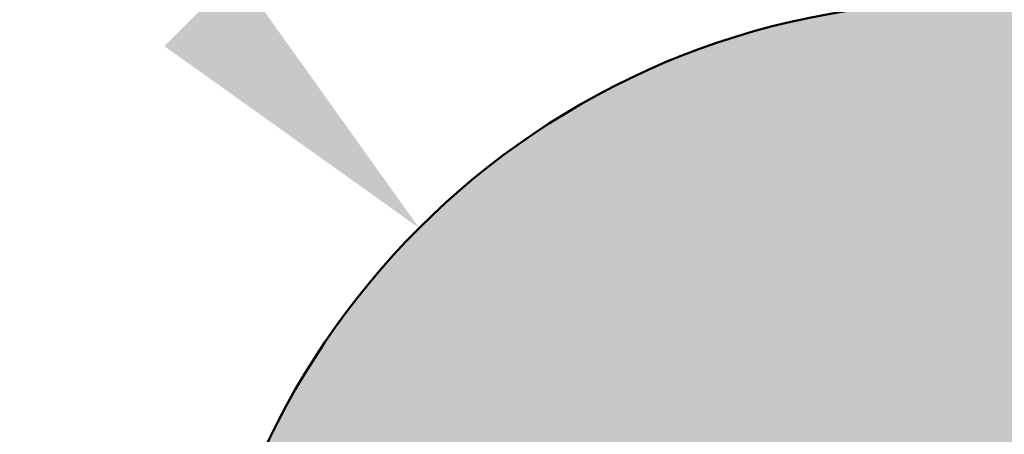
# Model space of a CAD drawing. Units: millimetres. Extents: x 0 to 2267, y 0 to 1823.
# Tile 15 of 256: x 1518.68 to 1531.44, y 1121.82 to 1127.19. Entities that reach past the tile are written whole.
import ezdxf

# ---------------------------------------------------------------- set-up
doc = ezdxf.new("R2010")
doc.units = ezdxf.units.MM
doc.header["$MEASUREMENT"] = 0
for name, color, linetype, lineweight in [('M-DIMS', 2, 'Continuous', 25), ('M-HATC', 252, 'Continuous', 18), ('M-OUTL', 7, 'Continuous', 50)]:
    doc.layers.add(name, color=color, linetype=linetype, lineweight=lineweight)
doc.styles.get("Standard").update_dxf_attribs({"font": 'arial.ttf'})
doc.dimstyles.get("Standard").update_dxf_attribs({"dimtxt": 7, "dimasz": 4, "dimexe": 0.18, "dimexo": 0.0625, "dimgap": 0.09, "dimtad": 0, "dimdec": 0, "dimzin": 0, "dimdsep": 46, "dimtxsty": 'Standard', "dimcen": 0.09, "dimadec": 0, "dimazin": 0, "dimtfac": 1, "dimtdec": 0, "dimtofl": 0, "dimtmove": 0, "dimatfit": 3, "dimfxl": 1, "dimtolj": 1, "dimtzin": 0, "dimarcsym": 0})

# ---------------------------------------------------------------- blocks, each defined once
blk = doc.blocks.new('*D28')
at = {"layer": 'Defpoints', "color": 0, "transparency": 16777216}
for p in [(1523.858, 1124.488), (1530.929, 1117.417)]:
    blk.add_point(p, dxfattribs=at)
at = {"layer": 'M-DIMS', "color": 0, "lineweight": -2, "transparency": 16777216}
for p, q in [((1518.201, 1130.145), (1521.029, 1127.317)), ((1530.839, 1117.417), (1531.019, 1117.417)), ((1530.929, 1117.327), (1530.929, 1117.507))]:
    blk.add_line(p, q, dxfattribs=at)
at = {"layer": 'M-DIMS', "color": 0, "transparency": 16777216}
blk.add_solid([(1521.501, 1127.788), (1520.558, 1126.845), (1523.858, 1124.488)], dxfattribs=at)
at = {"layer": 'M-DIMS', "color": 0, "transparency": 16777216, "insert": (1504.949, 1143.397), "char_height": 7, "attachment_point": 5, "rotation": 314.9998}
blk.add_mtext('\\A1;27X R10', dxfattribs=at)

msp = doc.modelspace()

# ---------------------------------------------------------------- hatches: boundary and pattern name
at = {"layer": 'M-HATC'}
h = msp.add_hatch(color=256, dxfattribs=at)
h.dxf.hatch_style = 1
h.paths.add_polyline_path([(2055.771, 1603.062), (1381.087, 1603.062), (1381.087, 1598.062), (2055.771, 1598.062)])
h.paths.add_polyline_path([(2055.771, 1598.062), (1381.087, 1598.062), (1381.087, 1593.062), (2055.771, 1593.062)])
h.paths.add_polyline_path([(2051.307, 1536.761), (1385.55, 1536.761), (1385.55, 1526.761), (1387.55, 1526.761), (1388.537, 1525.053), (1385.332, 1521.233), (1385.332, 1521.223), (2050.254, 1522.749), (2048.321, 1525.053), (2049.307, 1526.761), (2051.307, 1526.761)])
edge = h.paths.add_edge_path()
edge.add_arc((1847.535, 1379.149), 135, 222.60306, 222.89085, ccw=False)
edge.add_line((1748.166, 1287.766), (1683.092, 1287.766))
edge.add_arc((1583.724, 1379.149), 135, 317.10915, 317.39694, ccw=False)
edge.add_arc((1678.969, 1290.671), 5, 222.8909, 317.1091, ccw=False)
edge.add_arc((1774.213, 1379.149), 135, 222.60306, 222.89085, ccw=False)
edge.add_line((1674.845, 1287.766), (1609.771, 1287.766))
edge.add_arc((1510.403, 1379.149), 135, 317.10915, 317.39694, ccw=False)
edge.add_arc((1605.647, 1290.671), 5, 222.8909, 317.1091, ccw=False)
edge.add_arc((1700.892, 1379.149), 135, 222.60306, 222.89085, ccw=False)
edge.add_line((1601.524, 1287.766), (1536.45, 1287.766))
edge.add_arc((1437.081, 1379.149), 135, 317.10915, 317.39694, ccw=False)
edge.add_arc((1532.326, 1290.671), 5, 222.8909, 317.1091, ccw=False)
edge.add_arc((1627.571, 1379.149), 135, 222.60306, 222.89085, ccw=False)
edge.add_line((1528.203, 1287.766), (1505.929, 1287.766))
edge.add_spline(control_points=[(1505.929, 1287.766), (1504.262, 1287.766), (1504.262, 1282.766), (1505.929, 1282.766)], knot_values=[0, 0, 0, 0, 5, 5, 5, 5], degree=3, periodic=0)
edge.add_line((1505.929, 1282.766), (1930.929, 1282.766))
edge.add_spline(control_points=[(1930.929, 1282.766), (1932.596, 1282.766), (1932.596, 1287.766), (1930.929, 1287.766)], knot_values=[0, 0, 0, 0, 5, 5, 5, 5], degree=3, periodic=0)
edge.add_line((1930.929, 1287.766), (1903.056, 1287.766))
edge.add_arc((1803.688, 1379.149), 135, 317.10915, 317.39694, ccw=False)
edge.add_arc((1898.932, 1290.671), 5, 222.8909, 317.1091, ccw=False)
edge.add_arc((1994.177, 1379.149), 135, 222.60306, 222.89085, ccw=False)
edge.add_line((1894.809, 1287.766), (1829.735, 1287.766))
edge.add_arc((1730.366, 1379.149), 135, 317.10915, 317.39694, ccw=False)
edge.add_arc((1825.611, 1290.671), 5, 222.8909, 317.1091, ccw=False)
edge.add_arc((1920.856, 1379.149), 135, 222.60306, 222.89085, ccw=False)
edge.add_line((1821.487, 1287.766), (1756.413, 1287.766))
edge.add_arc((1657.045, 1379.149), 135, 317.10915, 317.39694, ccw=False)
edge.add_arc((1752.29, 1290.671), 5, 222.8909, 317.1091, ccw=False)
edge = h.paths.add_edge_path()
edge.add_spline(control_points=[(1843.429, 1227.247), (1845.096, 1227.247), (1845.096, 1232.247), (1843.429, 1232.247)], knot_values=[0, 0, 0, 0, 5, 5, 5, 5], degree=3, periodic=0)
edge.add_line((1843.429, 1232.247), (1593.429, 1232.247))
edge.add_spline(control_points=[(1593.429, 1232.247), (1591.762, 1232.247), (1591.762, 1227.247), (1593.429, 1227.247)], knot_values=[0, 0, 0, 0, 5, 5, 5, 5], degree=3, periodic=0)
edge.add_line((1593.429, 1227.247), (1843.429, 1227.247))
h.paths.add_polyline_path([(1905.929, 1127.417), (1530.929, 1127.417, 0.414214), (1520.929, 1117.417), (1530.929, 1117.417), (1915.929, 1117.417, 0.414214)])
edge = h.paths.add_edge_path()
edge.add_arc((1397.086, 1498.408), 12.73, 90.7821, 190.8787, ccw=False)
edge.add_line((1396.912, 1511.136), (1428.01, 1511.349))
edge.add_line((1428.01, 1511.349), (1433.01, 1511.349))
edge.add_line((1433.01, 1511.349), (1434.439, 1511.349))
edge.add_arc((1419.474, 1498.08), 20, 41.561, 74.0821)
edge.add_line((1424.959, 1517.314), (1399.935, 1517.256))
edge.add_spline(control_points=[(1399.931, 1517.256), (1399.884, 1517.213), (1399.833, 1517.169), (1399.777, 1517.124)], knot_values=[11.567499, 11.567499, 11.567499, 11.567499, 11.814249, 11.814249, 11.814249, 11.814249], degree=3, periodic=0)
edge.add_spline(control_points=[(1399.633, 1517.01), (1399.583, 1516.972), (1399.531, 1516.934), (1399.476, 1516.895)], knot_values=[11.167718, 11.167718, 11.167718, 11.167718, 11.365188, 11.365188, 11.365188, 11.365188], degree=3, periodic=0)
edge.add_spline(control_points=[(1399.34, 1516.8), (1399.151, 1516.672), (1398.938, 1516.538), (1398.704, 1516.399)], knot_values=[10.376405, 10.376405, 10.376405, 10.376405, 11.00994, 11.00994, 11.00994, 11.00994], degree=3, periodic=0)
edge.add_spline(control_points=[(1398.657, 1516.372), (1398.579, 1516.326), (1398.498, 1516.28), (1398.415, 1516.233)], knot_values=[10.125175, 10.125175, 10.125175, 10.125175, 10.334406, 10.334406, 10.334406, 10.334406], degree=3, periodic=0)
edge.add_spline(control_points=[(1398.264, 1516.149), (1398.196, 1516.111), (1398.126, 1516.073), (1398.055, 1516.035)], knot_values=[9.832246, 9.832246, 9.832246, 9.832246, 9.999658, 9.999658, 9.999658, 9.999658], degree=3, periodic=0)
edge.add_spline(control_points=[(1397.999, 1516.005), (1397.731, 1515.862), (1397.446, 1515.717), (1397.147, 1515.571)], knot_values=[9.161808, 9.161808, 9.161808, 9.161808, 9.787769, 9.787769, 9.787769, 9.787769], degree=3, periodic=0)
edge.add_spline(control_points=[(1397.147, 1515.571), (1396.842, 1515.423), (1396.522, 1515.274), (1396.191, 1515.126)], knot_values=[8.524455, 8.524455, 8.524455, 8.524455, 9.161808, 9.161808, 9.161808, 9.161808], degree=3, periodic=0)
edge.add_spline(control_points=[(1396.078, 1515.076), (1395.985, 1515.035), (1395.892, 1514.994), (1395.798, 1514.953)], knot_values=[8.275193, 8.275193, 8.275193, 8.275193, 8.451726, 8.451726, 8.451726, 8.451726], degree=3, periodic=0)
edge.add_spline(control_points=[(1395.602, 1514.869), (1395.5, 1514.826), (1395.397, 1514.782), (1395.293, 1514.739)], knot_values=[7.962917, 7.962917, 7.962917, 7.962917, 8.152764, 8.152764, 8.152764, 8.152764], degree=3, periodic=0)
edge.add_spline(control_points=[(1395.212, 1514.706), (1394.828, 1514.547), (1394.435, 1514.393), (1394.036, 1514.244)], knot_values=[7.21254, 7.21254, 7.21254, 7.21254, 7.913148, 7.913148, 7.913148, 7.913148], degree=3, periodic=0)
edge.add_spline(control_points=[(1394.036, 1514.244), (1393.708, 1514.121), (1393.375, 1514.003), (1393.043, 1513.889)], knot_values=[6.633733, 6.633733, 6.633733, 6.633733, 7.21254, 7.21254, 7.21254, 7.21254], degree=3, periodic=0)
edge.add_spline(control_points=[(1392.821, 1513.815), (1392.72, 1513.781), (1392.618, 1513.748), (1392.517, 1513.715)], knot_values=[6.328796, 6.328796, 6.328796, 6.328796, 6.505493, 6.505493, 6.505493, 6.505493], degree=3, periodic=0)
edge.add_spline(control_points=[(1392.517, 1513.715), (1392.319, 1513.652), (1392.121, 1513.59), (1391.924, 1513.531)], knot_values=[5.984605, 5.984605, 5.984605, 5.984605, 6.328796, 6.328796, 6.328796, 6.328796], degree=3, periodic=0)
edge.add_spline(control_points=[(1391.792, 1513.491), (1391.312, 1513.35), (1390.838, 1513.224), (1390.378, 1513.117)], knot_values=[5.066697, 5.066697, 5.066697, 5.066697, 5.907055, 5.907055, 5.907055, 5.907055], degree=3, periodic=0)
edge.add_spline(control_points=[(1390.378, 1513.117), (1390.18, 1513.071), (1389.984, 1513.028), (1389.791, 1512.99)], knot_values=[4.70367, 4.70367, 4.70367, 4.70367, 5.066695, 5.066695, 5.066695, 5.066695], degree=3, periodic=0)
edge.add_spline(control_points=[(1389.422, 1512.92), (1389.246, 1512.889), (1389.073, 1512.862), (1388.904, 1512.838)], knot_values=[4.130571, 4.130571, 4.130571, 4.130571, 4.469816, 4.469816, 4.469816, 4.469816], degree=3, periodic=0)
edge.add_spline(control_points=[(1388.904, 1512.838), (1388.591, 1512.795), (1388.291, 1512.764), (1388.007, 1512.749)], knot_values=[3.504031, 3.504031, 3.504031, 3.504031, 4.130571, 4.130571, 4.130571, 4.130571], degree=3, periodic=0)
edge.add_spline(control_points=[(1387.936, 1512.746), (1387.854, 1512.742), (1387.773, 1512.74), (1387.694, 1512.739)], knot_values=[3.268866, 3.268866, 3.268866, 3.268866, 3.451164, 3.451164, 3.451164, 3.451164], degree=3, periodic=0)
edge.add_spline(control_points=[(1387.335, 1512.744), (1387.208, 1512.75), (1387.085, 1512.76), (1386.967, 1512.774)], knot_values=[2.670686, 2.670686, 2.670686, 2.670686, 2.984, 2.984, 2.984, 2.984], degree=3, periodic=0)
edge.add_spline(control_points=[(1386.833, 1512.792), (1386.821, 1512.794), (1386.809, 1512.796), (1386.797, 1512.798)], knot_values=[2.516981, 2.516981, 2.516981, 2.516981, 2.549528, 2.549528, 2.549528, 2.549528], degree=3, periodic=0)
edge.add_spline(control_points=[(1386.453, 1512.873), (1386.426, 1512.881), (1386.399, 1512.889), (1386.373, 1512.897)], knot_values=[2.095869, 2.095869, 2.095869, 2.095869, 2.17941, 2.17941, 2.17941, 2.17941], degree=3, periodic=0)
edge.add_spline(control_points=[(1386.069, 1513.019), (1386.063, 1513.022), (1386.058, 1513.025), (1386.052, 1513.028)], knot_values=[1.72453, 1.72453, 1.72453, 1.72453, 1.745933, 1.745933, 1.745933, 1.745933], degree=3, periodic=0)
edge.add_arc((1399.474, 1498.08), 20, 131.8243, 180)
edge.add_arc((1630.334, 1505.548), 250.971, 181.70518, 236.42798)
edge.add_arc((1605.34, 1483.304), 218.782, 238.66083, 243.34961)
edge.add_arc((1647.091, 1510.359), 262.899, 183.12984, 237.85344, ccw=False)
h.paths.add_polyline_path([(1406.537, 1391.964, 0.149382), (1491.551, 1296.442, -0.129517)], flags=17)
edge = h.paths.add_edge_path()
edge.add_arc((2037.384, 1498.08), 20, 0, 48.2659)
edge.add_spline(control_points=[(2050.697, 1513.005), (2050.651, 1512.985), (2050.603, 1512.966), (2050.554, 1512.948)], knot_values=[1.835652, 1.835652, 1.835652, 1.835652, 2.000781, 2.000781, 2.000781, 2.000781], degree=3, periodic=0)
edge.add_spline(control_points=[(2050.462, 1512.917), (2050.479, 1512.922), (2050.496, 1512.928), (2050.513, 1512.934)], knot_values=[2.045477, 2.045477, 2.045477, 2.045477, 2.101389, 2.101389, 2.101389, 2.101389], degree=3, periodic=0)
edge.add_spline(control_points=[(2050.129, 1512.834), (2050.198, 1512.847), (2050.266, 1512.862), (2050.331, 1512.879)], knot_values=[2.237629, 2.237629, 2.237629, 2.237629, 2.435841, 2.435841, 2.435841, 2.435841], degree=3, periodic=0)
edge.add_spline(control_points=[(2050.095, 1512.828), (2050.106, 1512.83), (2050.118, 1512.832), (2050.129, 1512.834)], knot_values=[2.435841, 2.435841, 2.435841, 2.435841, 2.468321, 2.468321, 2.468321, 2.468321], degree=3, periodic=0)
edge.add_spline(control_points=[(2049.784, 1512.785), (2049.855, 1512.792), (2049.924, 1512.801), (2049.992, 1512.811)], knot_values=[2.563852, 2.563852, 2.563852, 2.563852, 2.748541, 2.748541, 2.748541, 2.748541], degree=3, periodic=0)
edge.add_spline(control_points=[(2049.405, 1512.762), (2049.536, 1512.765), (2049.663, 1512.773), (2049.784, 1512.785)], knot_values=[2.748541, 2.748541, 2.748541, 2.748541, 3.064882, 3.064882, 3.064882, 3.064882], degree=3, periodic=0)
edge.add_spline(control_points=[(2049.17, 1512.76), (2049.234, 1512.759), (2049.297, 1512.759), (2049.358, 1512.761)], knot_values=[3.102309, 3.102309, 3.102309, 3.102309, 3.2503, 3.2503, 3.2503, 3.2503], degree=3, periodic=0)
edge.add_spline(control_points=[(2048.857, 1512.769), (2048.964, 1512.764), (2049.068, 1512.761), (2049.17, 1512.76)], knot_values=[3.2503, 3.2503, 3.2503, 3.2503, 3.486069, 3.486069, 3.486069, 3.486069], degree=3, periodic=0)
edge.add_spline(control_points=[(2048.692, 1512.779), (2048.373, 1512.801), (2048.035, 1512.841), (2047.682, 1512.897)], knot_values=[3.606429, 3.606429, 3.606429, 3.606429, 4.2989, 4.2989, 4.2989, 4.2989], degree=3, periodic=0)
edge.add_spline(control_points=[(2047.682, 1512.897), (2047.546, 1512.919), (2047.408, 1512.942), (2047.268, 1512.969)], knot_values=[4.2989, 4.2989, 4.2989, 4.2989, 4.565769, 4.565769, 4.565769, 4.565769], degree=3, periodic=0)
edge.add_spline(control_points=[(2047.268, 1512.969), (2047.145, 1512.991), (2047.021, 1513.016), (2046.895, 1513.042)], knot_values=[4.565769, 4.565769, 4.565769, 4.565769, 4.799971, 4.799971, 4.799971, 4.799971], degree=3, periodic=0)
edge.add_spline(control_points=[(2046.895, 1513.042), (2046.529, 1513.119), (2046.151, 1513.209), (2045.768, 1513.311)], knot_values=[4.799971, 4.799971, 4.799971, 4.799971, 5.483718, 5.483718, 5.483718, 5.483718], degree=3, periodic=0)
edge.add_spline(control_points=[(2045.768, 1513.311), (2045.372, 1513.415), (2044.97, 1513.532), (2044.566, 1513.659)], knot_values=[5.483718, 5.483718, 5.483718, 5.483718, 6.187866, 6.187866, 6.187866, 6.187866], degree=3, periodic=0)
edge.add_spline(control_points=[(2044.566, 1513.659), (2044.415, 1513.706), (2044.263, 1513.755), (2044.112, 1513.805)], knot_values=[6.187866, 6.187866, 6.187866, 6.187866, 6.451551, 6.451551, 6.451551, 6.451551], degree=3, periodic=0)
edge.add_spline(control_points=[(2044.112, 1513.805), (2043.997, 1513.843), (2043.882, 1513.881), (2043.767, 1513.92)], knot_values=[6.451551, 6.451551, 6.451551, 6.451551, 6.651434, 6.651434, 6.651434, 6.651434], degree=3, periodic=0)
edge.add_spline(control_points=[(2043.767, 1513.92), (2043.372, 1514.055), (2042.977, 1514.198), (2042.589, 1514.346)], knot_values=[6.651434, 6.651434, 6.651434, 6.651434, 7.338879, 7.338879, 7.338879, 7.338879], degree=3, periodic=0)
edge.add_spline(control_points=[(2042.589, 1514.346), (2042.164, 1514.507), (2041.746, 1514.675), (2041.341, 1514.846)], knot_values=[7.338879, 7.338879, 7.338879, 7.338879, 8.089209, 8.089209, 8.089209, 8.089209], degree=3, periodic=0)
edge.add_spline(control_points=[(2041.341, 1514.846), (2041.103, 1514.946), (2040.869, 1515.048), (2040.64, 1515.15)], knot_values=[8.089209, 8.089209, 8.089209, 8.089209, 8.529587, 8.529587, 8.529587, 8.529587], degree=3, periodic=0)
edge.add_spline(control_points=[(2040.51, 1515.209), (2040.082, 1515.402), (2039.675, 1515.597), (2039.295, 1515.789)], knot_values=[8.613818, 8.613818, 8.613818, 8.613818, 9.44571, 9.44571, 9.44571, 9.44571], degree=3, periodic=0)
edge.add_spline(control_points=[(2039.295, 1515.789), (2039.062, 1515.907), (2038.839, 1516.025), (2038.629, 1516.14)], knot_values=[9.44571, 9.44571, 9.44571, 9.44571, 9.956404, 9.956404, 9.956404, 9.956404], degree=3, periodic=0)
edge.add_spline(control_points=[(2038.629, 1516.14), (2038.519, 1516.2), (2038.412, 1516.26), (2038.309, 1516.319)], knot_values=[9.956404, 9.956404, 9.956404, 9.956404, 10.223542, 10.223542, 10.223542, 10.223542], degree=3, periodic=0)
edge.add_spline(control_points=[(2038.309, 1516.319), (2038.214, 1516.374), (2038.122, 1516.428), (2038.033, 1516.481)], knot_values=[10.223542, 10.223542, 10.223542, 10.223542, 10.47051, 10.47051, 10.47051, 10.47051], degree=3, periodic=0)
edge.add_spline(control_points=[(2038.033, 1516.481), (2037.786, 1516.63), (2037.564, 1516.773), (2037.372, 1516.909)], knot_values=[10.47051, 10.47051, 10.47051, 10.47051, 11.15767, 11.15767, 11.15767, 11.15767], degree=3, periodic=0)
edge.add_spline(control_points=[(2037.372, 1516.909), (2037.279, 1516.975), (2037.193, 1517.04), (2037.114, 1517.102)], knot_values=[11.15767, 11.15767, 11.15767, 11.15767, 11.49227, 11.49227, 11.49227, 11.49227], degree=3, periodic=0)
edge.add_spline(control_points=[(2036.856, 1517.326), (2036.915, 1517.269), (2036.981, 1517.21), (2037.056, 1517.149)], knot_values=[11.577341, 11.577341, 11.577341, 11.577341, 11.91035, 11.91035, 11.91035, 11.91035], degree=3, periodic=0)
edge.add_spline(control_points=[(2036.807, 1517.375), (2036.823, 1517.359), (2036.839, 1517.342), (2036.856, 1517.326)], knot_values=[11.91035, 11.91035, 11.91035, 11.91035, 12.007402, 12.007402, 12.007402, 12.007402], degree=3, periodic=0)
edge.add_spline(control_points=[(2036.702, 1517.494), (2036.71, 1517.483), (2036.72, 1517.472), (2036.729, 1517.461)], knot_values=[12.184155, 12.184155, 12.184155, 12.184155, 12.255409, 12.255409, 12.255409, 12.255409], degree=3, periodic=0)
edge.add_spline(control_points=[(2036.616, 1517.621), (2036.62, 1517.613), (2036.624, 1517.606), (2036.629, 1517.598)], knot_values=[12.487913, 12.487913, 12.487913, 12.487913, 12.541035, 12.541035, 12.541035, 12.541035], degree=3, periodic=0)
edge.add_spline(control_points=[(2036.563, 1517.786), (2036.564, 1517.779), (2036.564, 1517.773), (2036.565, 1517.766)], knot_values=[12.911761, 12.911761, 12.911761, 12.911761, 12.968286, 12.968286, 12.968286, 12.968286], degree=3, periodic=0)
edge.add_spline(control_points=[(2036.617, 1517.93), (2036.612, 1517.926), (2036.609, 1517.921), (2036.605, 1517.916)], knot_values=[13.382527, 13.382527, 13.382527, 13.382527, 13.433791, 13.433791, 13.433791, 13.433791], degree=3, periodic=0)
edge.add_spline(control_points=[(2036.749, 1518.017), (2036.736, 1518.012), (2036.724, 1518.006), (2036.712, 1518)], knot_values=[13.726299, 13.726299, 13.726299, 13.726299, 13.809928, 13.809928, 13.809928, 13.809928], degree=3, periodic=0)
edge.add_spline(control_points=[(2036.86, 1518.053), (2036.839, 1518.047), (2036.818, 1518.042), (2036.799, 1518.035)], knot_values=[13.910887, 13.910887, 13.910887, 13.910887, 14.02153, 14.02153, 14.02153, 14.02153], degree=3, periodic=0)
edge.add_line((2036.964, 1518.08), (2032.384, 1518.08))
edge.add_line((2032.384, 1518.08), (2027.384, 1518.08))
edge.add_line((2027.384, 1518.08), (2022.384, 1518.08))
edge.add_line((2022.384, 1518.08), (2017.384, 1518.08))
edge.add_arc((2017.384, 1498.08), 20, 90, 138.439)
edge.add_line((2002.419, 1511.349), (2003.848, 1511.349))
edge.add_line((2003.848, 1511.349), (2008.848, 1511.349))
edge.add_line((2008.848, 1511.349), (2039.772, 1511.138))
edge.add_arc((2039.772, 1498.408), 12.73, -10.8787, 90, ccw=False)
edge.add_arc((1789.767, 1510.359), 262.899, 302.14656, 356.87016, ccw=False)
edge.add_arc((1831.518, 1483.304), 218.782, 296.65039, 301.33917)
edge.add_arc((1806.524, 1505.548), 250.971, 303.57202, 358.29482)
h.paths.add_polyline_path([(2030.321, 1391.964, -0.129517), (1945.307, 1296.442, 0.149382)], flags=17)
edge = h.paths.add_edge_path()
edge.add_spline(control_points=[(2037.246, 1518.082), (2037.29, 1518.081), (2037.336, 1518.08), (2037.384, 1518.08)], knot_values=[0.000012, 0.000012, 0.000012, 0.000012, 0.144754, 0.144754, 0.144754, 0.144754], degree=3, periodic=0)
edge.add_line((2037.336, 1518.08), (2037.01, 1518.08))
edge.add_spline(control_points=[(2037.01, 1518.08), (2036.982, 1518.077), (2036.956, 1518.073), (2036.931, 1518.068)], knot_values=[14.13465, 14.13465, 14.13465, 14.13465, 14.247197, 14.247197, 14.247197, 14.247197], degree=3, periodic=0)
edge.add_spline(control_points=[(2036.931, 1518.068), (2036.928, 1518.067), (2036.924, 1518.067), (2036.921, 1518.066)], knot_values=[14.118315, 14.118315, 14.118315, 14.118315, 14.13465, 14.13465, 14.13465, 14.13465], degree=3, periodic=0)
edge.add_spline(control_points=[(2036.921, 1518.066), (2036.912, 1518.064), (2036.903, 1518.063), (2036.895, 1518.061)], knot_values=[14.078086, 14.078086, 14.078086, 14.078086, 14.118315, 14.118315, 14.118315, 14.118315], degree=3, periodic=0)
edge.add_spline(control_points=[(2036.895, 1518.061), (2036.883, 1518.058), (2036.872, 1518.056), (2036.86, 1518.053)], knot_values=[14.02153, 14.02153, 14.02153, 14.02153, 14.078086, 14.078086, 14.078086, 14.078086], degree=3, periodic=0)
edge.add_spline(control_points=[(2036.86, 1518.053), (2036.839, 1518.047), (2036.818, 1518.042), (2036.799, 1518.035)], knot_values=[13.910887, 13.910887, 13.910887, 13.910887, 14.02153, 14.02153, 14.02153, 14.02153], degree=3, periodic=0)
edge.add_spline(control_points=[(2036.799, 1518.035), (2036.798, 1518.035), (2036.797, 1518.035), (2036.797, 1518.035)], knot_values=[13.906906, 13.906906, 13.906906, 13.906906, 13.910887, 13.910887, 13.910887, 13.910887], degree=3, periodic=0)
edge.add_spline(control_points=[(2036.797, 1518.035), (2036.788, 1518.032), (2036.78, 1518.029), (2036.772, 1518.026)], knot_values=[13.857826, 13.857826, 13.857826, 13.857826, 13.906906, 13.906906, 13.906906, 13.906906], degree=3, periodic=0)
edge.add_spline(control_points=[(2036.772, 1518.026), (2036.764, 1518.023), (2036.756, 1518.02), (2036.749, 1518.017)], knot_values=[13.809928, 13.809928, 13.809928, 13.809928, 13.857826, 13.857826, 13.857826, 13.857826], degree=3, periodic=0)
edge.add_spline(control_points=[(2036.749, 1518.017), (2036.736, 1518.012), (2036.724, 1518.006), (2036.712, 1518)], knot_values=[13.726299, 13.726299, 13.726299, 13.726299, 13.809928, 13.809928, 13.809928, 13.809928], degree=3, periodic=0)
edge.add_spline(control_points=[(2036.712, 1518), (2036.712, 1518), (2036.712, 1518), (2036.711, 1518)], knot_values=[13.723993, 13.723993, 13.723993, 13.723993, 13.726299, 13.726299, 13.726299, 13.726299], degree=3, periodic=0)
edge.add_spline(control_points=[(2036.711, 1518), (2036.706, 1517.997), (2036.701, 1517.994), (2036.696, 1517.992)], knot_values=[13.686536, 13.686536, 13.686536, 13.686536, 13.723993, 13.723993, 13.723993, 13.723993], degree=3, periodic=0)
edge.add_spline(control_points=[(2036.696, 1517.992), (2036.692, 1517.989), (2036.687, 1517.987), (2036.683, 1517.984)], knot_values=[13.651251, 13.651251, 13.651251, 13.651251, 13.686536, 13.686536, 13.686536, 13.686536], degree=3, periodic=0)
edge.add_spline(control_points=[(2036.683, 1517.984), (2036.676, 1517.98), (2036.67, 1517.976), (2036.664, 1517.971)], knot_values=[13.596804, 13.596804, 13.596804, 13.596804, 13.651251, 13.651251, 13.651251, 13.651251], degree=3, periodic=0)
edge.add_spline(control_points=[(2036.664, 1517.971), (2036.664, 1517.971), (2036.663, 1517.971), (2036.663, 1517.971)], knot_values=[13.593956, 13.593956, 13.593956, 13.593956, 13.596804, 13.596804, 13.596804, 13.596804], degree=3, periodic=0)
edge.add_spline(control_points=[(2036.663, 1517.971), (2036.66, 1517.969), (2036.658, 1517.967), (2036.655, 1517.965)], knot_values=[13.570322, 13.570322, 13.570322, 13.570322, 13.593956, 13.593956, 13.593956, 13.593956], degree=3, periodic=0)
edge.add_spline(control_points=[(2036.655, 1517.965), (2036.653, 1517.963), (2036.65, 1517.961), (2036.647, 1517.959)], knot_values=[13.545477, 13.545477, 13.545477, 13.545477, 13.570322, 13.570322, 13.570322, 13.570322], degree=3, periodic=0)
edge.add_spline(control_points=[(2036.647, 1517.959), (2036.647, 1517.959), (2036.647, 1517.959), (2036.647, 1517.959)], knot_values=[13.543931, 13.543931, 13.543931, 13.543931, 13.545477, 13.545477, 13.545477, 13.545477], degree=3, periodic=0)
edge.add_spline(control_points=[(2036.647, 1517.959), (2036.641, 1517.954), (2036.636, 1517.949), (2036.631, 1517.945)], knot_values=[13.488237, 13.488237, 13.488237, 13.488237, 13.543931, 13.543931, 13.543931, 13.543931], degree=3, periodic=0)
edge.add_spline(control_points=[(2036.631, 1517.945), (2036.628, 1517.942), (2036.626, 1517.94), (2036.623, 1517.937)], knot_values=[13.460307, 13.460307, 13.460307, 13.460307, 13.488237, 13.488237, 13.488237, 13.488237], degree=3, periodic=0)
edge.add_spline(control_points=[(2036.623, 1517.937), (2036.622, 1517.936), (2036.62, 1517.934), (2036.618, 1517.932)], knot_values=[13.439712, 13.439712, 13.439712, 13.439712, 13.460307, 13.460307, 13.460307, 13.460307], degree=3, periodic=0)
edge.add_spline(control_points=[(2036.618, 1517.932), (2036.618, 1517.931), (2036.617, 1517.931), (2036.617, 1517.93)], knot_values=[13.433791, 13.433791, 13.433791, 13.433791, 13.439712, 13.439712, 13.439712, 13.439712], degree=3, periodic=0)
edge.add_spline(control_points=[(2036.617, 1517.93), (2036.612, 1517.926), (2036.609, 1517.921), (2036.605, 1517.916)], knot_values=[13.382527, 13.382527, 13.382527, 13.382527, 13.433791, 13.433791, 13.433791, 13.433791], degree=3, periodic=0)
edge.add_spline(control_points=[(2036.605, 1517.916), (2036.603, 1517.913), (2036.6, 1517.91), (2036.598, 1517.907)], knot_values=[13.350017, 13.350017, 13.350017, 13.350017, 13.382527, 13.382527, 13.382527, 13.382527], degree=3, periodic=0)
edge.add_spline(control_points=[(2036.598, 1517.907), (2036.597, 1517.906), (2036.596, 1517.904), (2036.595, 1517.903)], knot_values=[13.333922, 13.333922, 13.333922, 13.333922, 13.350017, 13.350017, 13.350017, 13.350017], degree=3, periodic=0)
edge.add_spline(control_points=[(2036.595, 1517.903), (2036.595, 1517.902), (2036.594, 1517.901), (2036.593, 1517.9)], knot_values=[13.323828, 13.323828, 13.323828, 13.323828, 13.333922, 13.333922, 13.333922, 13.333922], degree=3, periodic=0)
edge.add_spline(control_points=[(2036.593, 1517.9), (2036.59, 1517.895), (2036.588, 1517.891), (2036.585, 1517.886)], knot_values=[13.277545, 13.277545, 13.277545, 13.277545, 13.323828, 13.323828, 13.323828, 13.323828], degree=3, periodic=0)
edge.add_spline(control_points=[(2036.585, 1517.886), (2036.584, 1517.883), (2036.582, 1517.879), (2036.58, 1517.875)], knot_values=[13.240119, 13.240119, 13.240119, 13.240119, 13.277545, 13.277545, 13.277545, 13.277545], degree=3, periodic=0)
edge.add_spline(control_points=[(2036.58, 1517.875), (2036.58, 1517.874), (2036.579, 1517.873), (2036.578, 1517.872)], knot_values=[13.228211, 13.228211, 13.228211, 13.228211, 13.240119, 13.240119, 13.240119, 13.240119], degree=3, periodic=0)
edge.add_spline(control_points=[(2036.578, 1517.872), (2036.578, 1517.87), (2036.577, 1517.869), (2036.577, 1517.868)], knot_values=[13.215717, 13.215717, 13.215717, 13.215717, 13.228211, 13.228211, 13.228211, 13.228211], degree=3, periodic=0)
edge.add_spline(control_points=[(2036.577, 1517.868), (2036.575, 1517.864), (2036.574, 1517.86), (2036.573, 1517.857)], knot_values=[13.179847, 13.179847, 13.179847, 13.179847, 13.215717, 13.215717, 13.215717, 13.215717], degree=3, periodic=0)
edge.add_spline(control_points=[(2036.573, 1517.857), (2036.571, 1517.851), (2036.57, 1517.846), (2036.569, 1517.841)], knot_values=[13.132017, 13.132017, 13.132017, 13.132017, 13.179847, 13.179847, 13.179847, 13.179847], degree=3, periodic=0)
edge.add_spline(control_points=[(2036.569, 1517.841), (2036.568, 1517.84), (2036.568, 1517.839), (2036.568, 1517.838)], knot_values=[13.122482, 13.122482, 13.122482, 13.122482, 13.132017, 13.132017, 13.132017, 13.132017], degree=3, periodic=0)
edge.add_spline(control_points=[(2036.568, 1517.838), (2036.568, 1517.836), (2036.567, 1517.835), (2036.567, 1517.833)], knot_values=[13.105592, 13.105592, 13.105592, 13.105592, 13.122482, 13.122482, 13.122482, 13.122482], degree=3, periodic=0)
edge.add_spline(control_points=[(2036.567, 1517.833), (2036.566, 1517.829), (2036.566, 1517.826), (2036.565, 1517.822)], knot_values=[13.074063, 13.074063, 13.074063, 13.074063, 13.105592, 13.105592, 13.105592, 13.105592], degree=3, periodic=0)
edge.add_spline(control_points=[(2036.565, 1517.822), (2036.565, 1517.822), (2036.565, 1517.822), (2036.565, 1517.822)], knot_values=[13.074043, 13.074043, 13.074043, 13.074043, 13.074063, 13.074063, 13.074063, 13.074063], degree=3, periodic=0)
edge.add_spline(control_points=[(2036.565, 1517.822), (2036.564, 1517.816), (2036.564, 1517.811), (2036.564, 1517.805)], knot_values=[13.021884, 13.021884, 13.021884, 13.021884, 13.074043, 13.074043, 13.074043, 13.074043], degree=3, periodic=0)
edge.add_spline(control_points=[(2036.564, 1517.805), (2036.564, 1517.804), (2036.564, 1517.803), (2036.564, 1517.803)], knot_values=[13.01674, 13.01674, 13.01674, 13.01674, 13.021884, 13.021884, 13.021884, 13.021884], degree=3, periodic=0)
edge.add_spline(control_points=[(2036.564, 1517.803), (2036.563, 1517.801), (2036.563, 1517.798), (2036.563, 1517.796)], knot_values=[12.996438, 12.996438, 12.996438, 12.996438, 13.01674, 13.01674, 13.01674, 13.01674], degree=3, periodic=0)
edge.add_spline(control_points=[(2036.563, 1517.796), (2036.563, 1517.793), (2036.563, 1517.789), (2036.563, 1517.786)], knot_values=[12.968286, 12.968286, 12.968286, 12.968286, 12.996438, 12.996438, 12.996438, 12.996438], degree=3, periodic=0)
edge.add_spline(control_points=[(2036.563, 1517.786), (2036.564, 1517.779), (2036.564, 1517.773), (2036.565, 1517.766)], knot_values=[12.911761, 12.911761, 12.911761, 12.911761, 12.968286, 12.968286, 12.968286, 12.968286], degree=3, periodic=0)
edge.add_spline(control_points=[(2036.565, 1517.766), (2036.565, 1517.766), (2036.565, 1517.766), (2036.565, 1517.766)], knot_values=[12.911017, 12.911017, 12.911017, 12.911017, 12.911761, 12.911761, 12.911761, 12.911761], degree=3, periodic=0)
edge.add_spline(control_points=[(2036.565, 1517.766), (2036.565, 1517.762), (2036.566, 1517.759), (2036.566, 1517.756)], knot_values=[12.88528, 12.88528, 12.88528, 12.88528, 12.911017, 12.911017, 12.911017, 12.911017], degree=3, periodic=0)
edge.add_spline(control_points=[(2036.566, 1517.756), (2036.567, 1517.753), (2036.567, 1517.751), (2036.568, 1517.748)], knot_values=[12.862519, 12.862519, 12.862519, 12.862519, 12.88528, 12.88528, 12.88528, 12.88528], degree=3, periodic=0)
edge.add_spline(control_points=[(2036.568, 1517.748), (2036.568, 1517.747), (2036.568, 1517.747), (2036.568, 1517.746)], knot_values=[12.858885, 12.858885, 12.858885, 12.858885, 12.862519, 12.862519, 12.862519, 12.862519], degree=3, periodic=0)
edge.add_spline(control_points=[(2036.568, 1517.746), (2036.569, 1517.74), (2036.571, 1517.733), (2036.572, 1517.726)], knot_values=[12.8053, 12.8053, 12.8053, 12.8053, 12.858885, 12.858885, 12.858885, 12.858885], degree=3, periodic=0)
edge.add_spline(control_points=[(2036.572, 1517.726), (2036.573, 1517.723), (2036.574, 1517.719), (2036.576, 1517.715)], knot_values=[12.775176, 12.775176, 12.775176, 12.775176, 12.8053, 12.8053, 12.8053, 12.8053], degree=3, periodic=0)
edge.add_spline(control_points=[(2036.576, 1517.715), (2036.576, 1517.713), (2036.577, 1517.71), (2036.578, 1517.708)], knot_values=[12.756759, 12.756759, 12.756759, 12.756759, 12.775176, 12.775176, 12.775176, 12.775176], degree=3, periodic=0)
edge.add_spline(control_points=[(2036.578, 1517.708), (2036.578, 1517.707), (2036.578, 1517.706), (2036.579, 1517.705)], knot_values=[12.748742, 12.748742, 12.748742, 12.748742, 12.756759, 12.756759, 12.756759, 12.756759], degree=3, periodic=0)
edge.add_spline(control_points=[(2036.579, 1517.705), (2036.581, 1517.698), (2036.583, 1517.692), (2036.586, 1517.685)], knot_values=[12.69959, 12.69959, 12.69959, 12.69959, 12.748742, 12.748742, 12.748742, 12.748742], degree=3, periodic=0)
edge.add_spline(control_points=[(2036.586, 1517.685), (2036.588, 1517.68), (2036.59, 1517.675), (2036.592, 1517.669)], knot_values=[12.659038, 12.659038, 12.659038, 12.659038, 12.69959, 12.69959, 12.69959, 12.69959], degree=3, periodic=0)
edge.add_spline(control_points=[(2036.592, 1517.669), (2036.594, 1517.665), (2036.596, 1517.66), (2036.598, 1517.656)], knot_values=[12.626806, 12.626806, 12.626806, 12.626806, 12.659038, 12.659038, 12.659038, 12.659038], degree=3, periodic=0)
edge.add_spline(control_points=[(2036.598, 1517.656), (2036.598, 1517.655), (2036.599, 1517.654), (2036.599, 1517.653)], knot_values=[12.619394, 12.619394, 12.619394, 12.619394, 12.626806, 12.626806, 12.626806, 12.626806], degree=3, periodic=0)
edge.add_spline(control_points=[(2036.599, 1517.653), (2036.604, 1517.642), (2036.61, 1517.632), (2036.616, 1517.621)], knot_values=[12.541039, 12.541039, 12.541039, 12.541039, 12.619394, 12.619394, 12.619394, 12.619394], degree=3, periodic=0)
edge.add_spline(control_points=[(2036.616, 1517.621), (2036.616, 1517.621), (2036.616, 1517.621), (2036.616, 1517.621)], knot_values=[12.541035, 12.541035, 12.541035, 12.541035, 12.541039, 12.541039, 12.541039, 12.541039], degree=3, periodic=0)
edge.add_spline(control_points=[(2036.616, 1517.621), (2036.62, 1517.613), (2036.624, 1517.606), (2036.629, 1517.598)], knot_values=[12.487913, 12.487913, 12.487913, 12.487913, 12.541035, 12.541035, 12.541035, 12.541035], degree=3, periodic=0)
edge.add_spline(control_points=[(2036.629, 1517.598), (2036.633, 1517.592), (2036.637, 1517.585), (2036.641, 1517.579)], knot_values=[12.443982, 12.443982, 12.443982, 12.443982, 12.487913, 12.487913, 12.487913, 12.487913], degree=3, periodic=0)
edge.add_spline(control_points=[(2036.641, 1517.579), (2036.641, 1517.578), (2036.642, 1517.576), (2036.643, 1517.575)], knot_values=[12.434996, 12.434996, 12.434996, 12.434996, 12.443982, 12.443982, 12.443982, 12.443982], degree=3, periodic=0)
edge.add_spline(control_points=[(2036.643, 1517.575), (2036.653, 1517.56), (2036.664, 1517.544), (2036.676, 1517.528)], knot_values=[12.329647, 12.329647, 12.329647, 12.329647, 12.434996, 12.434996, 12.434996, 12.434996], degree=3, periodic=0)
edge.add_spline(control_points=[(2036.676, 1517.528), (2036.684, 1517.517), (2036.693, 1517.505), (2036.702, 1517.494)], knot_values=[12.255409, 12.255409, 12.255409, 12.255409, 12.329647, 12.329647, 12.329647, 12.329647], degree=3, periodic=0)
edge.add_spline(control_points=[(2036.702, 1517.494), (2036.71, 1517.483), (2036.72, 1517.472), (2036.729, 1517.461)], knot_values=[12.184155, 12.184155, 12.184155, 12.184155, 12.255409, 12.255409, 12.255409, 12.255409], degree=3, periodic=0)
edge.add_spline(control_points=[(2036.729, 1517.461), (2036.744, 1517.444), (2036.759, 1517.426), (2036.775, 1517.409)], knot_values=[12.075961, 12.075961, 12.075961, 12.075961, 12.184155, 12.184155, 12.184155, 12.184155], degree=3, periodic=0)
edge.add_spline(control_points=[(2036.775, 1517.409), (2036.776, 1517.407), (2036.777, 1517.406), (2036.778, 1517.405)], knot_values=[12.069502, 12.069502, 12.069502, 12.069502, 12.075961, 12.075961, 12.075961, 12.075961], degree=3, periodic=0)
edge.add_spline(control_points=[(2036.778, 1517.405), (2036.788, 1517.395), (2036.797, 1517.385), (2036.807, 1517.375)], knot_values=[12.007402, 12.007402, 12.007402, 12.007402, 12.069502, 12.069502, 12.069502, 12.069502], degree=3, periodic=0)
edge.add_spline(control_points=[(2036.807, 1517.375), (2036.823, 1517.359), (2036.839, 1517.342), (2036.856, 1517.326)], knot_values=[11.91035, 11.91035, 11.91035, 11.91035, 12.007402, 12.007402, 12.007402, 12.007402], degree=3, periodic=0)
edge.add_spline(control_points=[(2036.856, 1517.326), (2036.915, 1517.269), (2036.981, 1517.21), (2037.056, 1517.149)], knot_values=[11.577341, 11.577341, 11.577341, 11.577341, 11.91035, 11.91035, 11.91035, 11.91035], degree=3, periodic=0)
edge.add_spline(control_points=[(2037.056, 1517.149), (2037.075, 1517.134), (2037.094, 1517.118), (2037.114, 1517.102)], knot_values=[11.49227, 11.49227, 11.49227, 11.49227, 11.577341, 11.577341, 11.577341, 11.577341], degree=3, periodic=0)
edge.add_spline(control_points=[(2037.114, 1517.102), (2037.193, 1517.04), (2037.279, 1516.975), (2037.372, 1516.909)], knot_values=[11.15767, 11.15767, 11.15767, 11.15767, 11.49227, 11.49227, 11.49227, 11.49227], degree=3, periodic=0)
edge.add_spline(control_points=[(2037.372, 1516.909), (2037.564, 1516.773), (2037.786, 1516.63), (2038.033, 1516.481)], knot_values=[10.47051, 10.47051, 10.47051, 10.47051, 11.15767, 11.15767, 11.15767, 11.15767], degree=3, periodic=0)
edge.add_spline(control_points=[(2038.033, 1516.481), (2038.122, 1516.428), (2038.214, 1516.374), (2038.309, 1516.319)], knot_values=[10.223542, 10.223542, 10.223542, 10.223542, 10.47051, 10.47051, 10.47051, 10.47051], degree=3, periodic=0)
edge.add_spline(control_points=[(2038.309, 1516.319), (2038.412, 1516.26), (2038.519, 1516.2), (2038.629, 1516.14)], knot_values=[9.956404, 9.956404, 9.956404, 9.956404, 10.223542, 10.223542, 10.223542, 10.223542], degree=3, periodic=0)
edge.add_spline(control_points=[(2038.629, 1516.14), (2038.839, 1516.025), (2039.062, 1515.907), (2039.295, 1515.789)], knot_values=[9.44571, 9.44571, 9.44571, 9.44571, 9.956404, 9.956404, 9.956404, 9.956404], degree=3, periodic=0)
edge.add_spline(control_points=[(2039.295, 1515.789), (2039.675, 1515.597), (2040.082, 1515.402), (2040.51, 1515.209)], knot_values=[8.613818, 8.613818, 8.613818, 8.613818, 9.44571, 9.44571, 9.44571, 9.44571], degree=3, periodic=0)
edge.add_spline(control_points=[(2040.51, 1515.209), (2040.553, 1515.189), (2040.597, 1515.17), (2040.64, 1515.15)], knot_values=[8.529587, 8.529587, 8.529587, 8.529587, 8.613818, 8.613818, 8.613818, 8.613818], degree=3, periodic=0)
edge.add_spline(control_points=[(2040.64, 1515.15), (2040.869, 1515.048), (2041.103, 1514.946), (2041.341, 1514.846)], knot_values=[8.089209, 8.089209, 8.089209, 8.089209, 8.529587, 8.529587, 8.529587, 8.529587], degree=3, periodic=0)
edge.add_spline(control_points=[(2041.341, 1514.846), (2041.746, 1514.675), (2042.164, 1514.507), (2042.589, 1514.346)], knot_values=[7.338879, 7.338879, 7.338879, 7.338879, 8.089209, 8.089209, 8.089209, 8.089209], degree=3, periodic=0)
edge.add_spline(control_points=[(2042.589, 1514.346), (2042.977, 1514.198), (2043.372, 1514.055), (2043.767, 1513.92)], knot_values=[6.651434, 6.651434, 6.651434, 6.651434, 7.338879, 7.338879, 7.338879, 7.338879], degree=3, periodic=0)
edge.add_spline(control_points=[(2043.767, 1513.92), (2043.882, 1513.881), (2043.997, 1513.843), (2044.112, 1513.805)], knot_values=[6.451551, 6.451551, 6.451551, 6.451551, 6.651434, 6.651434, 6.651434, 6.651434], degree=3, periodic=0)
edge.add_spline(control_points=[(2044.112, 1513.805), (2044.263, 1513.755), (2044.415, 1513.706), (2044.566, 1513.659)], knot_values=[6.187866, 6.187866, 6.187866, 6.187866, 6.451551, 6.451551, 6.451551, 6.451551], degree=3, periodic=0)
edge.add_spline(control_points=[(2044.566, 1513.659), (2044.97, 1513.532), (2045.372, 1513.415), (2045.768, 1513.311)], knot_values=[5.483718, 5.483718, 5.483718, 5.483718, 6.187866, 6.187866, 6.187866, 6.187866], degree=3, periodic=0)
edge.add_spline(control_points=[(2045.768, 1513.311), (2046.151, 1513.209), (2046.529, 1513.119), (2046.895, 1513.042)], knot_values=[4.799971, 4.799971, 4.799971, 4.799971, 5.483718, 5.483718, 5.483718, 5.483718], degree=3, periodic=0)
edge.add_spline(control_points=[(2046.895, 1513.042), (2047.021, 1513.016), (2047.145, 1512.991), (2047.268, 1512.969)], knot_values=[4.565769, 4.565769, 4.565769, 4.565769, 4.799971, 4.799971, 4.799971, 4.799971], degree=3, periodic=0)
edge.add_spline(control_points=[(2047.268, 1512.969), (2047.408, 1512.942), (2047.546, 1512.919), (2047.682, 1512.897)], knot_values=[4.2989, 4.2989, 4.2989, 4.2989, 4.565769, 4.565769, 4.565769, 4.565769], degree=3, periodic=0)
edge.add_spline(control_points=[(2047.682, 1512.897), (2048.035, 1512.841), (2048.373, 1512.801), (2048.692, 1512.779)], knot_values=[3.606429, 3.606429, 3.606429, 3.606429, 4.2989, 4.2989, 4.2989, 4.2989], degree=3, periodic=0)
edge.add_spline(control_points=[(2048.692, 1512.779), (2048.748, 1512.775), (2048.803, 1512.772), (2048.857, 1512.769)], knot_values=[3.486069, 3.486069, 3.486069, 3.486069, 3.606429, 3.606429, 3.606429, 3.606429], degree=3, periodic=0)
edge.add_spline(control_points=[(2048.857, 1512.769), (2048.964, 1512.764), (2049.068, 1512.761), (2049.17, 1512.76)], knot_values=[3.2503, 3.2503, 3.2503, 3.2503, 3.486069, 3.486069, 3.486069, 3.486069], degree=3, periodic=0)
edge.add_spline(control_points=[(2049.17, 1512.76), (2049.234, 1512.759), (2049.297, 1512.759), (2049.358, 1512.761)], knot_values=[3.102309, 3.102309, 3.102309, 3.102309, 3.2503, 3.2503, 3.2503, 3.2503], degree=3, periodic=0)
edge.add_spline(control_points=[(2049.358, 1512.761), (2049.374, 1512.761), (2049.39, 1512.761), (2049.405, 1512.762)], knot_values=[3.064882, 3.064882, 3.064882, 3.064882, 3.102309, 3.102309, 3.102309, 3.102309], degree=3, periodic=0)
edge.add_spline(control_points=[(2049.405, 1512.762), (2049.536, 1512.765), (2049.663, 1512.773), (2049.784, 1512.785)], knot_values=[2.748541, 2.748541, 2.748541, 2.748541, 3.064882, 3.064882, 3.064882, 3.064882], degree=3, periodic=0)
edge.add_spline(control_points=[(2049.784, 1512.785), (2049.855, 1512.792), (2049.924, 1512.801), (2049.992, 1512.811)], knot_values=[2.563852, 2.563852, 2.563852, 2.563852, 2.748541, 2.748541, 2.748541, 2.748541], degree=3, periodic=0)
edge.add_spline(control_points=[(2049.992, 1512.811), (2050.026, 1512.816), (2050.061, 1512.822), (2050.095, 1512.828)], knot_values=[2.468321, 2.468321, 2.468321, 2.468321, 2.563852, 2.563852, 2.563852, 2.563852], degree=3, periodic=0)
edge.add_spline(control_points=[(2050.095, 1512.828), (2050.106, 1512.83), (2050.118, 1512.832), (2050.129, 1512.834)], knot_values=[2.435841, 2.435841, 2.435841, 2.435841, 2.468321, 2.468321, 2.468321, 2.468321], degree=3, periodic=0)
edge.add_spline(control_points=[(2050.129, 1512.834), (2050.198, 1512.847), (2050.266, 1512.862), (2050.331, 1512.879)], knot_values=[2.237629, 2.237629, 2.237629, 2.237629, 2.435841, 2.435841, 2.435841, 2.435841], degree=3, periodic=0)
edge.add_spline(control_points=[(2050.331, 1512.879), (2050.375, 1512.891), (2050.419, 1512.903), (2050.462, 1512.917)], knot_values=[2.101389, 2.101389, 2.101389, 2.101389, 2.237629, 2.237629, 2.237629, 2.237629], degree=3, periodic=0)
edge.add_spline(control_points=[(2050.462, 1512.917), (2050.479, 1512.922), (2050.496, 1512.928), (2050.513, 1512.934)], knot_values=[2.045477, 2.045477, 2.045477, 2.045477, 2.101389, 2.101389, 2.101389, 2.101389], degree=3, periodic=0)
edge.add_spline(control_points=[(2050.513, 1512.934), (2050.527, 1512.938), (2050.54, 1512.943), (2050.554, 1512.948)], knot_values=[2.000781, 2.000781, 2.000781, 2.000781, 2.045477, 2.045477, 2.045477, 2.045477], degree=3, periodic=0)
edge.add_spline(control_points=[(2050.554, 1512.948), (2050.603, 1512.966), (2050.651, 1512.985), (2050.697, 1513.005)], knot_values=[1.835652, 1.835652, 1.835652, 1.835652, 2.000781, 2.000781, 2.000781, 2.000781], degree=3, periodic=0)
edge.add_arc((2037.384, 1498.08), 20, 48.2659, 90.1299)
edge = h.paths.add_edge_path(flags=16)
edge.add_spline(control_points=[(1386.139, 1512.986), (1388.92, 1511.739), (1398.039, 1515.519), (1399.931, 1517.256)], knot_values=[1.831046, 1.831046, 1.831046, 1.831046, 11.814249, 11.814249, 11.814249, 11.814249], degree=3, periodic=0)
edge.add_line((1399.931, 1517.256), (1393.743, 1517.242))
edge.add_arc((1399.474, 1498.08), 20, 106.6501, 131.8173)

# ---------------------------------------------------------------- linework, layer by layer
at = {"layer": 'M-OUTL'}
msp.add_arc((1530.929, 1117.417), 10, 90, 180, dxfattribs=at)

# ---------------------------------------------------------------- dimensions: what is measured, and where the dimension line sits
at = {"layer": 'M-DIMS'}
dim = msp.add_radius_dim(center=(1530.929, 1117.417), mpoint=(1523.858, 1124.488), text='27X <>', dimstyle='Standard', override={"dimdec": 0, "dimlfac": 1, "dimrnd": 0, "dimzin": 0, "dimdsep": 46, "dimlunit": 2}, dxfattribs=at)
dim.commit()
dim.dimension.update_dxf_attribs({"geometry": '*D28', "text_midpoint": (1504.949, 1143.397)})

doc.saveas('drawing.dxf')
